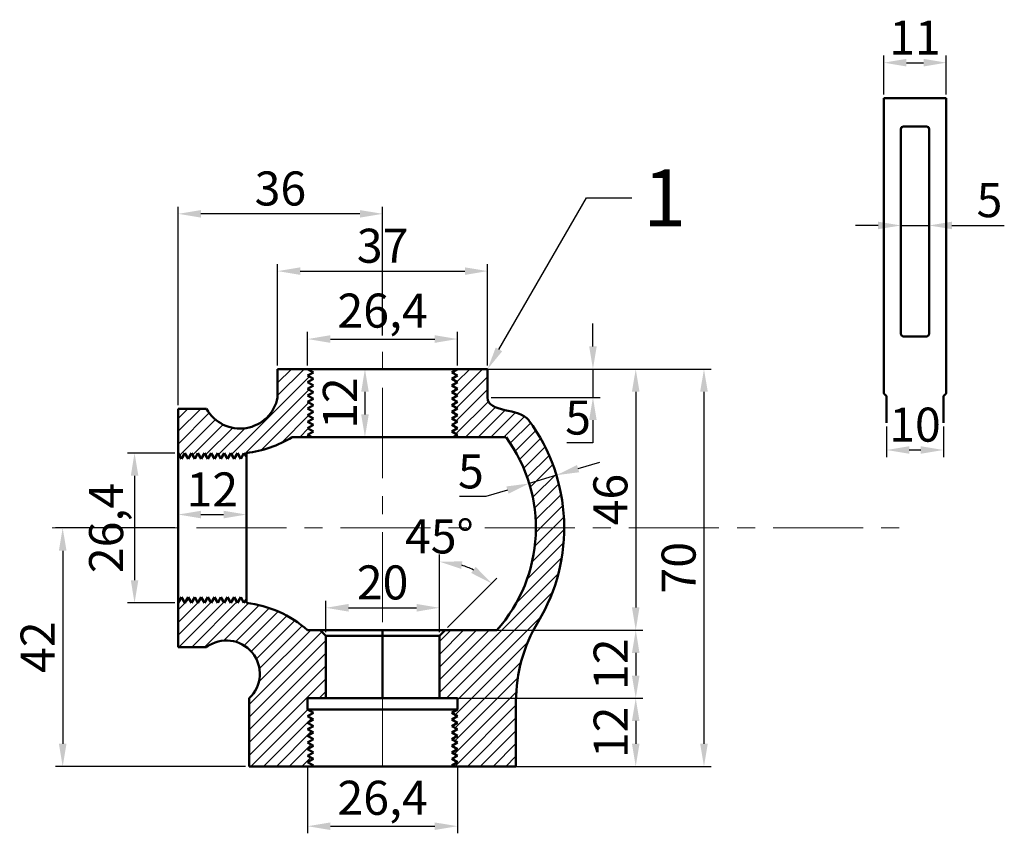
# Model space of a CAD drawing. Units: millimetres. Extents: x -25 to 763, y -62 to 306.
# Tile 3 of 7: x 266 to 439, y 32 to 175. Entities that reach past the tile are written whole.
import ezdxf
from ezdxf import colors
from ezdxf.entities.mleader import LeaderData, LeaderLine
from ezdxf.math import Vec2, Vec3

# ---------------------------------------------------------------- set-up
doc = ezdxf.new("R2010")
doc.units = ezdxf.units.MM
doc.header["$LTSCALE"] = 0.5
doc.linetypes.add('CENTER', pattern=[50.8, 31.75, -6.35, 6.35, -6.35])
for name, color, linetype, lineweight in [('M-CNTR', 1, 'CENTER', 18), ('M-DIMS', 2, 'Continuous', 25), ('M-HATC', 8, 'Continuous', 18), ('M-OUTL', 7, 'Continuous', 50), ('M-TEXT', 3, 'Continuous', 25)]:
    doc.layers.add(name, color=color, linetype=linetype, lineweight=lineweight)
doc.styles.get("Standard").update_dxf_attribs({"font": 'arial.ttf'})
doc.dimstyles.new('ISO-25', dxfattribs={"dimtxt": 6, "dimasz": 4, "dimexe": 1.25, "dimexo": 0.625, "dimtad": 1, "dimtoh": 1, "dimdec": 1, "dimtxsty": 'Standard', "dimcen": 2.5, "dimadec": 0, "dimazin": 0, "dimtfac": 1, "dimtdec": 1, "dimtmove": 0, "dimatfit": 3, "dimfxl": 1, "dimarcsym": 0})

# ---------------------------------------------------------------- blocks, each defined once
blk = doc.blocks.new('*D1')
at = {"layer": 'Defpoints', "color": 0, "ltscale": 0.5, "transparency": 16777216}
for p in [(293.54, 98.87), (285.84, 72.47), (293.54, 72.47)]:
    blk.add_point(p, dxfattribs=at)
at = {"layer": 'M-DIMS', "color": 0, "lineweight": -2, "ltscale": 0.5, "transparency": 16777216}
for p, q in [((292.91, 98.87), (284.59, 98.87)), ((285.84, 94.87), (285.84, 76.47)), ((292.91, 72.47), (284.59, 72.47))]:
    blk.add_line(p, q, dxfattribs=at)
at = {"layer": 'M-DIMS', "color": 0, "ltscale": 0.5, "transparency": 16777216}
for points in [[(285.18, 94.87), (286.51, 94.87), (285.84, 98.87)], [(285.18, 76.47), (286.51, 76.47), (285.84, 72.47)]]:
    blk.add_solid(points, dxfattribs=at)
at = {"layer": 'M-DIMS', "color": 0, "ltscale": 0.5, "transparency": 16777216, "insert": (281.61, 85.67), "char_height": 6, "attachment_point": 5, "rotation": 90}
blk.add_mtext('26,4', dxfattribs=at)
blk = doc.blocks.new('*D2')
at = {"layer": 'Defpoints', "color": 0, "ltscale": 0.5, "transparency": 16777216}
for p in [(293.54, 85.67), (273.18, 43.67), (306.04, 43.67)]:
    blk.add_point(p, dxfattribs=at)
at = {"layer": 'M-DIMS', "color": 0, "lineweight": -2, "ltscale": 0.5, "transparency": 16777216}
for p, q in [((292.91, 85.67), (271.93, 85.67)), ((273.18, 81.67), (273.18, 47.67)), ((305.41, 43.67), (271.93, 43.67))]:
    blk.add_line(p, q, dxfattribs=at)
at = {"layer": 'M-DIMS', "color": 0, "ltscale": 0.5, "transparency": 16777216}
for points in [[(272.51, 81.67), (273.85, 81.67), (273.18, 85.67)], [(272.51, 47.67), (273.85, 47.67), (273.18, 43.67)]]:
    blk.add_solid(points, dxfattribs=at)
at = {"layer": 'M-DIMS', "color": 0, "ltscale": 0.5, "transparency": 16777216, "insert": (269.54, 64.67), "char_height": 6, "attachment_point": 5, "rotation": 90}
blk.add_mtext('42', dxfattribs=at)
blk = doc.blocks.new('*D3')
at = {"layer": 'Defpoints', "color": 0, "ltscale": 0.5, "transparency": 16777216}
for p in [(305.54, 88.04), (293.54, 85.67), (305.54, 85.67)]:
    blk.add_point(p, dxfattribs=at)
at = {"layer": 'M-DIMS', "color": 0, "lineweight": -2, "ltscale": 0.5, "transparency": 16777216}
for p, q in [((293.54, 86.3), (293.54, 89.29)), ((305.54, 86.3), (305.54, 89.29)), ((297.54, 88.04), (301.54, 88.04))]:
    blk.add_line(p, q, dxfattribs=at)
at = {"layer": 'M-DIMS', "color": 0, "ltscale": 0.5, "transparency": 16777216}
for points in [[(297.54, 88.7), (297.54, 87.37), (293.54, 88.04)], [(301.54, 88.7), (301.54, 87.37), (305.54, 88.04)]]:
    blk.add_solid(points, dxfattribs=at)
at = {"layer": 'M-DIMS', "color": 0, "ltscale": 0.5, "transparency": 16777216, "insert": (299.54, 91.68), "char_height": 6, "attachment_point": 5}
blk.add_mtext('12', dxfattribs=at)
blk = doc.blocks.new('*D4')
at = {"layer": 'Defpoints', "color": 0, "ltscale": 0.5, "transparency": 16777216}
for p in [(316.34, 44.4), (342.74, 44.4), (342.74, 33.13)]:
    blk.add_point(p, dxfattribs=at)
at = {"layer": 'M-DIMS', "color": 0, "lineweight": -2, "ltscale": 0.5, "transparency": 16777216}
for p, q in [((316.34, 43.77), (316.34, 31.88)), ((342.74, 43.77), (342.74, 31.88)), ((320.34, 33.13), (338.74, 33.13))]:
    blk.add_line(p, q, dxfattribs=at)
at = {"layer": 'M-DIMS', "color": 0, "ltscale": 0.5, "transparency": 16777216}
for points in [[(320.34, 33.79), (320.34, 32.46), (316.34, 33.13)], [(338.74, 33.79), (338.74, 32.46), (342.74, 33.13)]]:
    blk.add_solid(points, dxfattribs=at)
at = {"layer": 'M-DIMS', "color": 0, "ltscale": 0.5, "transparency": 16777216, "insert": (329.54, 37.36), "char_height": 6, "attachment_point": 5}
blk.add_mtext('26,4', dxfattribs=at)
blk = doc.blocks.new('*D5')
at = {"layer": 'Defpoints', "color": 0, "ltscale": 0.5, "transparency": 16777216}
for p in [(342.74, 55.67), (344.97, 43.67), (374.14, 43.67)]:
    blk.add_point(p, dxfattribs=at)
at = {"layer": 'M-DIMS', "color": 0, "lineweight": -2, "ltscale": 0.5, "transparency": 16777216}
for p, q in [((343.36, 55.67), (375.39, 55.67)), ((374.14, 51.67), (374.14, 47.67)), ((345.6, 43.67), (375.39, 43.67))]:
    blk.add_line(p, q, dxfattribs=at)
at = {"layer": 'M-DIMS', "color": 0, "ltscale": 0.5, "transparency": 16777216}
for points in [[(373.47, 51.67), (374.8, 51.67), (374.14, 55.67)], [(373.47, 47.67), (374.8, 47.67), (374.14, 43.67)]]:
    blk.add_solid(points, dxfattribs=at)
at = {"layer": 'M-DIMS', "color": 0, "ltscale": 0.5, "transparency": 16777216, "insert": (370.5, 49.67), "char_height": 6, "attachment_point": 5, "rotation": 90}
blk.add_mtext('12', dxfattribs=at)
blk = doc.blocks.new('*D6')
at = {"layer": 'Defpoints', "color": 0, "ltscale": 0.5, "transparency": 16777216}
for p in [(339.54, 67.67), (339.54, 55.67), (374.14, 55.67)]:
    blk.add_point(p, dxfattribs=at)
at = {"layer": 'M-DIMS', "color": 0, "lineweight": -2, "ltscale": 0.5, "transparency": 16777216}
for p, q in [((340.16, 67.67), (375.39, 67.67)), ((374.14, 63.67), (374.14, 59.67)), ((340.16, 55.67), (375.39, 55.67))]:
    blk.add_line(p, q, dxfattribs=at)
at = {"layer": 'M-DIMS', "color": 0, "ltscale": 0.5, "transparency": 16777216}
for points in [[(373.47, 63.67), (374.8, 63.67), (374.14, 67.67)], [(373.47, 59.67), (374.8, 59.67), (374.14, 55.67)]]:
    blk.add_solid(points, dxfattribs=at)
at = {"layer": 'M-DIMS', "color": 0, "ltscale": 0.5, "transparency": 16777216, "insert": (370.5, 61.67), "char_height": 6, "attachment_point": 5, "rotation": 90}
blk.add_mtext('12', dxfattribs=at)
blk = doc.blocks.new('*D7')
at = {"layer": 'Defpoints', "color": 0, "ltscale": 0.5, "transparency": 16777216}
for p in [(346.51, 113.67), (346.51, 67.67), (374.14, 67.67)]:
    blk.add_point(p, dxfattribs=at)
at = {"layer": 'M-DIMS', "color": 0, "lineweight": -2, "ltscale": 0.5, "transparency": 16777216}
for p, q in [((347.13, 113.67), (375.39, 113.67)), ((374.14, 109.67), (374.14, 71.67)), ((347.13, 67.67), (375.39, 67.67))]:
    blk.add_line(p, q, dxfattribs=at)
at = {"layer": 'M-DIMS', "color": 0, "ltscale": 0.5, "transparency": 16777216}
for points in [[(373.47, 109.67), (374.8, 109.67), (374.14, 113.67)], [(373.47, 71.67), (374.8, 71.67), (374.14, 67.67)]]:
    blk.add_solid(points, dxfattribs=at)
at = {"layer": 'M-DIMS', "color": 0, "ltscale": 0.5, "transparency": 16777216, "insert": (370.45, 90.67), "char_height": 6, "attachment_point": 5, "rotation": 90}
blk.add_mtext('46', dxfattribs=at)
blk = doc.blocks.new('*D8')
at = {"layer": 'Defpoints', "color": 0, "ltscale": 0.5, "transparency": 16777216}
for p in [(361.26, 113.67), (361.26, 43.67), (386.16, 43.67)]:
    blk.add_point(p, dxfattribs=at)
at = {"layer": 'M-DIMS', "color": 0, "lineweight": -2, "ltscale": 0.5, "transparency": 16777216}
for p, q in [((361.89, 113.67), (387.41, 113.67)), ((386.16, 109.67), (386.16, 47.67)), ((361.89, 43.67), (387.41, 43.67))]:
    blk.add_line(p, q, dxfattribs=at)
at = {"layer": 'M-DIMS', "color": 0, "ltscale": 0.5, "transparency": 16777216}
for points in [[(385.49, 109.67), (386.83, 109.67), (386.16, 113.67)], [(385.49, 47.67), (386.83, 47.67), (386.16, 43.67)]]:
    blk.add_solid(points, dxfattribs=at)
at = {"layer": 'M-DIMS', "color": 0, "ltscale": 0.5, "transparency": 16777216, "insert": (382.47, 78.67), "char_height": 6, "attachment_point": 5, "rotation": 90}
blk.add_mtext('70', dxfattribs=at)
blk = doc.blocks.new('*D9')
at = {"layer": 'Defpoints', "color": 0, "ltscale": 0.5, "transparency": 16777216}
for p in [(360.16, 94.97), (355.37, 93.51), (355.37, 93.51)]:
    blk.add_point(p, dxfattribs=at)
at = {"layer": 'M-DIMS', "color": 0, "lineweight": -2, "ltscale": 0.5, "transparency": 16777216}
for p, q in [((363.98, 96.13), (367.81, 97.29)), ((359.97, 95.57), (359.79, 96.16)), ((355.19, 94.11), (355.01, 94.71)), ((360.16, 94.97), (355.37, 93.51)), ((351.54, 92.35), (347.72, 91.19)), ((347.72, 91.19), (343.11, 91.19))]:
    blk.add_line(p, q, dxfattribs=at)
at = {"layer": 'M-DIMS', "color": 0, "ltscale": 0.5, "transparency": 16777216}
for points in [[(363.79, 96.77), (364.18, 95.49), (360.16, 94.97)], [(351.35, 92.99), (351.74, 91.72), (355.37, 93.51)]]:
    blk.add_solid(points, dxfattribs=at)
at = {"layer": 'M-DIMS', "color": 0, "ltscale": 0.5, "transparency": 16777216, "insert": (345.1, 94.87), "char_height": 6, "attachment_point": 5}
blk.add_mtext('5', dxfattribs=at)
blk = doc.blocks.new('*D10')
at = {"layer": 'Defpoints', "color": 0, "ltscale": 0.5, "transparency": 16777216}
for p in [(339.54, 71.61), (319.54, 66.67), (339.54, 66.67)]:
    blk.add_point(p, dxfattribs=at)
at = {"layer": 'M-DIMS', "color": 0, "lineweight": -2, "ltscale": 0.5, "transparency": 16777216}
for p, q in [((319.54, 67.3), (319.54, 72.86)), ((339.54, 67.3), (339.54, 72.86)), ((323.54, 71.61), (335.54, 71.61))]:
    blk.add_line(p, q, dxfattribs=at)
at = {"layer": 'M-DIMS', "color": 0, "ltscale": 0.5, "transparency": 16777216}
for points in [[(323.54, 72.28), (323.54, 70.94), (319.54, 71.61)], [(335.54, 72.28), (335.54, 70.94), (339.54, 71.61)]]:
    blk.add_solid(points, dxfattribs=at)
at = {"layer": 'M-DIMS', "color": 0, "ltscale": 0.5, "transparency": 16777216, "insert": (329.54, 75.3), "char_height": 6, "attachment_point": 5}
blk.add_mtext('20', dxfattribs=at)
blk = doc.blocks.new('*D11')
at = {"layer": 'Defpoints', "color": 0, "ltscale": 0.5, "transparency": 16777216}
for p in [(346.07, 77.99), (340.54, 67.67), (339.54, 66.67), (339.54, 66.67), (339.54, 55.67)]:
    blk.add_point(p, dxfattribs=at)
at = {"layer": 'M-DIMS', "color": 0, "lineweight": -2, "ltscale": 0.5, "transparency": 16777216}
for p, q in [((339.54, 67.3), (339.54, 80.99)), ((340.98, 68.11), (349.66, 76.8))]:
    blk.add_line(p, q, dxfattribs=at)
blk.add_arc((339.54, 66.67), 13.06, 62.6113, 72.3887, dxfattribs=at)
at = {"layer": 'M-DIMS', "color": 0, "ltscale": 0.5, "transparency": 16777216}
for points in [[(343.39, 78.47), (343.59, 79.78), (339.54, 79.74)], [(345.94, 78.81), (345.15, 77.74), (348.77, 75.91)]]:
    blk.add_solid(points, dxfattribs=at)
at = {"layer": 'M-DIMS', "color": 0, "ltscale": 0.5, "transparency": 16777216, "insert": (339.54, 83.41), "char_height": 6, "attachment_point": 5}
blk.add_mtext('45°', dxfattribs=at)
blk = doc.blocks.new('*D12')
at = {"layer": 'Defpoints', "color": 0, "ltscale": 0.5, "transparency": 16777216}
for p in [(293.54, 141.02), (329.54, 118.96), (293.54, 106.67)]:
    blk.add_point(p, dxfattribs=at)
at = {"layer": 'M-DIMS', "color": 0, "lineweight": -2, "ltscale": 0.5, "transparency": 16777216}
for p, q in [((293.54, 107.3), (293.54, 142.27)), ((329.54, 119.59), (329.54, 142.27)), ((325.54, 141.02), (297.54, 141.02))]:
    blk.add_line(p, q, dxfattribs=at)
at = {"layer": 'M-DIMS', "color": 0, "ltscale": 0.5, "transparency": 16777216}
for points in [[(297.54, 141.68), (297.54, 140.35), (293.54, 141.02)], [(325.54, 141.68), (325.54, 140.35), (329.54, 141.02)]]:
    blk.add_solid(points, dxfattribs=at)
at = {"layer": 'M-DIMS', "color": 0, "ltscale": 0.5, "transparency": 16777216, "insert": (311.54, 144.71), "char_height": 6, "attachment_point": 5}
blk.add_mtext('36', dxfattribs=at)
blk = doc.blocks.new('*D13')
at = {"layer": 'Defpoints', "color": 0, "ltscale": 0.5, "transparency": 16777216}
for p in [(348.04, 130.93), (311.04, 113.67), (348.04, 113.67)]:
    blk.add_point(p, dxfattribs=at)
at = {"layer": 'M-DIMS', "color": 0, "lineweight": -2, "ltscale": 0.5, "transparency": 16777216}
for p, q in [((311.04, 114.3), (311.04, 132.18)), ((348.04, 114.3), (348.04, 132.18)), ((315.04, 130.93), (344.04, 130.93))]:
    blk.add_line(p, q, dxfattribs=at)
at = {"layer": 'M-DIMS', "color": 0, "ltscale": 0.5, "transparency": 16777216}
for points in [[(315.04, 131.59), (315.04, 130.26), (311.04, 130.93)], [(344.04, 131.59), (344.04, 130.26), (348.04, 130.93)]]:
    blk.add_solid(points, dxfattribs=at)
at = {"layer": 'M-DIMS', "color": 0, "ltscale": 0.5, "transparency": 16777216, "insert": (329.54, 134.62), "char_height": 6, "attachment_point": 5}
blk.add_mtext('37', dxfattribs=at)
blk = doc.blocks.new('*D14')
at = {"layer": 'Defpoints', "color": 0, "ltscale": 0.5, "transparency": 16777216}
for p in [(342.74, 118.96), (316.34, 113.67), (342.74, 113.67)]:
    blk.add_point(p, dxfattribs=at)
at = {"layer": 'M-DIMS', "color": 0, "lineweight": -2, "ltscale": 0.5, "transparency": 16777216}
for p, q in [((316.34, 114.3), (316.34, 120.21)), ((342.74, 114.3), (342.74, 120.21)), ((320.34, 118.96), (338.74, 118.96))]:
    blk.add_line(p, q, dxfattribs=at)
at = {"layer": 'M-DIMS', "color": 0, "ltscale": 0.5, "transparency": 16777216}
for points in [[(320.34, 119.63), (320.34, 118.29), (316.34, 118.96)], [(338.74, 119.63), (338.74, 118.29), (342.74, 118.96)]]:
    blk.add_solid(points, dxfattribs=at)
at = {"layer": 'M-DIMS', "color": 0, "ltscale": 0.5, "transparency": 16777216, "insert": (329.54, 123.19), "char_height": 6, "attachment_point": 5}
blk.add_mtext('26,4', dxfattribs=at)
blk = doc.blocks.new('*D15')
at = {"layer": 'Defpoints', "color": 0, "ltscale": 0.5, "transparency": 16777216}
for p in [(329.54, 113.67), (326.43, 101.67), (329.54, 101.67)]:
    blk.add_point(p, dxfattribs=at)
at = {"layer": 'M-DIMS', "color": 0, "lineweight": -2, "ltscale": 0.5, "transparency": 16777216}
for p, q in [((328.91, 113.67), (325.18, 113.67)), ((326.43, 109.67), (326.43, 105.67)), ((328.91, 101.67), (325.18, 101.67))]:
    blk.add_line(p, q, dxfattribs=at)
at = {"layer": 'M-DIMS', "color": 0, "ltscale": 0.5, "transparency": 16777216}
for points in [[(325.77, 109.67), (327.1, 109.67), (326.43, 113.67)], [(325.77, 105.67), (327.1, 105.67), (326.43, 101.67)]]:
    blk.add_solid(points, dxfattribs=at)
at = {"layer": 'M-DIMS', "color": 0, "ltscale": 0.5, "transparency": 16777216, "insert": (322.8, 107.67), "char_height": 6, "attachment_point": 5, "rotation": 90}
blk.add_mtext('12', dxfattribs=at)
blk = doc.blocks.new('*D16')
at = {"layer": 'Defpoints', "color": 0, "ltscale": 0.5, "transparency": 16777216}
for p in [(348.04, 113.67), (348.04, 108.67), (366.6, 108.67)]:
    blk.add_point(p, dxfattribs=at)
at = {"layer": 'M-DIMS', "color": 0, "lineweight": -2, "ltscale": 0.5, "transparency": 16777216}
for p, q in [((366.6, 117.67), (366.6, 121.67)), ((348.66, 113.67), (367.85, 113.67)), ((366.6, 113.67), (366.6, 108.67)), ((348.66, 108.67), (367.85, 108.67)), ((366.6, 104.67), (366.6, 100.67)), ((366.6, 100.67), (361.99, 100.67))]:
    blk.add_line(p, q, dxfattribs=at)
at = {"layer": 'M-DIMS', "color": 0, "ltscale": 0.5, "transparency": 16777216}
for points in [[(365.93, 117.67), (367.26, 117.67), (366.6, 113.67)], [(365.93, 104.67), (367.26, 104.67), (366.6, 108.67)]]:
    blk.add_solid(points, dxfattribs=at)
at = {"layer": 'M-DIMS', "color": 0, "ltscale": 0.5, "transparency": 16777216, "insert": (363.98, 104.35), "char_height": 6, "attachment_point": 5}
blk.add_mtext('5', dxfattribs=at)
blk = doc.blocks.new('*D19')
at = {"layer": 'Defpoints', "color": 0, "ltscale": 0.5, "transparency": 16777216}
for p in [(428.84, 167.65), (417.84, 161.41), (428.84, 161.41)]:
    blk.add_point(p, dxfattribs=at)
at = {"layer": 'M-DIMS', "color": 0, "lineweight": -2, "ltscale": 0.5, "transparency": 16777216}
for p, q in [((417.84, 162.04), (417.84, 168.9)), ((428.84, 162.04), (428.84, 168.9)), ((421.84, 167.65), (424.84, 167.65))]:
    blk.add_line(p, q, dxfattribs=at)
at = {"layer": 'M-DIMS', "color": 0, "ltscale": 0.5, "transparency": 16777216}
for points in [[(421.84, 168.32), (421.84, 166.98), (417.84, 167.65)], [(424.84, 168.32), (424.84, 166.98), (428.84, 167.65)]]:
    blk.add_solid(points, dxfattribs=at)
at = {"layer": 'M-DIMS', "color": 0, "ltscale": 0.5, "transparency": 16777216, "insert": (423.34, 171.29), "char_height": 6, "attachment_point": 5}
blk.add_mtext('11', dxfattribs=at)
blk = doc.blocks.new('*D20')
at = {"layer": 'Defpoints', "color": 0, "ltscale": 0.5, "transparency": 16777216}
for p in [(425.84, 138.97), (420.84, 137.91), (425.84, 137.91)]:
    blk.add_point(p, dxfattribs=at)
at = {"layer": 'M-DIMS', "color": 0, "lineweight": -2, "ltscale": 0.5, "transparency": 16777216}
for p, q in [((416.84, 138.97), (412.84, 138.97)), ((420.84, 138.54), (420.84, 140.22)), ((420.84, 138.97), (425.84, 138.97)), ((425.84, 138.54), (425.84, 140.22)), ((429.84, 138.97), (439.07, 138.97))]:
    blk.add_line(p, q, dxfattribs=at)
at = {"layer": 'M-DIMS', "color": 0, "ltscale": 0.5, "transparency": 16777216}
for points in [[(416.84, 139.64), (416.84, 138.31), (420.84, 138.97)], [(429.84, 139.64), (429.84, 138.31), (425.84, 138.97)]]:
    blk.add_solid(points, dxfattribs=at)
at = {"layer": 'M-DIMS', "color": 0, "ltscale": 0.5, "transparency": 16777216, "insert": (436.46, 142.65), "char_height": 6, "attachment_point": 5}
blk.add_mtext('5', dxfattribs=at)
blk = doc.blocks.new('*D21')
at = {"layer": 'Defpoints', "color": 0, "ltscale": 0.5, "transparency": 16777216}
for p in [(418.34, 104.19), (428.34, 104.19), (428.34, 99.41)]:
    blk.add_point(p, dxfattribs=at)
at = {"layer": 'M-DIMS', "color": 0, "lineweight": -2, "ltscale": 0.5, "transparency": 16777216}
for p, q in [((418.34, 103.57), (418.34, 98.16)), ((428.34, 103.57), (428.34, 98.16)), ((422.34, 99.41), (424.34, 99.41))]:
    blk.add_line(p, q, dxfattribs=at)
at = {"layer": 'M-DIMS', "color": 0, "ltscale": 0.5, "transparency": 16777216}
for points in [[(422.34, 100.08), (422.34, 98.74), (418.34, 99.41)], [(424.34, 100.08), (424.34, 98.74), (428.34, 99.41)]]:
    blk.add_solid(points, dxfattribs=at)
at = {"layer": 'M-DIMS', "color": 0, "ltscale": 0.5, "transparency": 16777216, "insert": (423.34, 103.1), "char_height": 6, "attachment_point": 5}
blk.add_mtext('10', dxfattribs=at)

msp = doc.modelspace()

# ---------------------------------------------------------------- hatches: boundary and pattern name
at = {"layer": 'M-HATC', "ltscale": 0.5}
h = msp.add_hatch(dxfattribs=at)
h.set_pattern_fill('ANSI31', color=256, scale=0.5)
h.paths.add_polyline_path([(305.54, 72.47), (305.54, 73.17), (305.12, 72.47), (304.54, 73.47), (303.97, 72.47), (303.39, 73.47), (302.81, 72.47), (302.24, 73.47), (301.64, 72.47), (301.07, 73.47), (300.49, 72.47), (299.91, 73.47), (299.34, 72.47), (298.76, 73.47), (298.17, 72.47), (297.59, 73.47), (297.01, 72.47), (296.44, 73.47), (295.86, 72.47), (295.28, 73.47), (294.69, 72.47), (294.11, 73.47), (293.54, 72.47), (293.54, 64.67), (298.54, 64.67, -0.948835), (306.04, 55.67), (306.04, 43.67), (317.08, 43.67), (317.34, 43.82), (316.34, 44.4), (317.34, 44.97), (316.34, 45.55), (317.34, 46.13), (316.34, 46.72), (317.34, 47.3), (316.34, 47.87), (317.34, 48.45), (316.34, 49.03), (317.34, 49.61), (316.34, 50.2), (317.34, 50.77), (316.34, 51.35), (317.34, 51.93), (316.34, 52.51), (317.34, 53.08), (316.34, 53.67), (316.34, 55.67), (319.54, 55.67), (319.54, 66.67), (318.54, 67.67), (316.34, 67.67, 0.150651)])
h.paths.add_polyline_path([(302.81, 98.87), (303.39, 97.87), (303.97, 98.87), (304.54, 97.87), (305.12, 98.87), (305.54, 98.17), (305.54, 98.87, 0.107745), (313.61, 101.67), (317.03, 101.67), (316.34, 102.07), (317.34, 102.65), (316.34, 103.24), (317.34, 103.82), (316.34, 104.4), (317.34, 104.97), (316.34, 105.55), (317.34, 106.13), (316.34, 106.72), (317.34, 107.3), (316.34, 107.87), (317.34, 108.45), (316.34, 109.03), (317.34, 109.61), (316.34, 110.2), (317.34, 110.77), (316.34, 111.35), (317.34, 111.93), (316.34, 112.51), (317.34, 113.08), (316.34, 113.67), (311.04, 113.67), (311.04, 108.67, -0.702826), (298.54, 106.67), (293.54, 106.67), (293.54, 98.87), (294.11, 97.87), (294.69, 98.87), (295.28, 97.87), (295.86, 98.87), (296.44, 97.87), (297.01, 98.87), (297.59, 97.87), (298.17, 98.87), (298.76, 97.87), (299.34, 98.87), (299.91, 97.87), (300.49, 98.87), (301.07, 97.87), (301.64, 98.87), (302.24, 97.87)])
edge = h.paths.add_edge_path()
edge.add_arc((329.54, 85.67), 27, 0, 36.3412, ccw=False)
edge.add_line((356.54, 85.67), (361.54, 85.67))
edge.add_arc((329.54, 85.67), 32, 0, 36.3412)
edge.add_spline(control_points=[(355.31, 104.64), (353.67, 106.87), (348.04, 105.9), (348.04, 108.67)], knot_values=[0, 0, 0, 0, 8.320994, 8.320994, 8.320994, 8.320994], degree=3, periodic=0)
edge.add_line((348.04, 108.67), (348.04, 113.67))
edge.add_line((348.04, 113.67), (342.74, 113.67))
edge.add_line((342.74, 113.67), (341.74, 113.08))
edge.add_line((341.74, 113.08), (342.74, 112.51))
edge.add_line((342.74, 112.51), (341.74, 111.93))
edge.add_line((341.74, 111.93), (342.74, 111.35))
edge.add_line((342.74, 111.35), (341.74, 110.77))
edge.add_line((341.74, 110.77), (342.74, 110.2))
edge.add_line((342.74, 110.2), (341.74, 109.61))
edge.add_line((341.74, 109.61), (342.74, 109.03))
edge.add_line((342.74, 109.03), (341.74, 108.45))
edge.add_line((341.74, 108.45), (342.74, 107.87))
edge.add_line((342.74, 107.87), (341.74, 107.3))
edge.add_line((341.74, 107.3), (342.74, 106.72))
edge.add_line((342.74, 106.72), (341.74, 106.13))
edge.add_line((341.74, 106.13), (342.74, 105.55))
edge.add_line((342.74, 105.55), (341.74, 104.97))
edge.add_line((341.74, 104.97), (342.74, 104.4))
edge.add_line((342.74, 104.4), (341.74, 103.82))
edge.add_line((341.74, 103.82), (342.74, 103.24))
edge.add_line((342.74, 103.24), (341.74, 102.65))
edge.add_line((341.74, 102.65), (342.74, 102.07))
edge.add_line((342.74, 102.07), (342.04, 101.67))
edge.add_line((342.04, 101.67), (351.28, 101.67))
h.paths.add_polyline_path([(349.66, 67.67), (340.54, 67.67), (339.54, 66.67), (339.54, 55.67), (342.74, 55.67), (342.74, 53.67), (341.74, 53.08), (342.74, 52.51), (341.74, 51.93), (342.74, 51.35), (341.74, 50.77), (342.74, 50.2), (341.74, 49.61), (342.74, 49.03), (341.74, 48.45), (342.74, 47.87), (341.74, 47.3), (342.74, 46.72), (341.74, 46.13), (342.74, 45.55), (341.74, 44.97), (342.74, 44.4), (341.74, 43.82), (341.99, 43.67), (353.04, 43.67), (353.04, 55.16, -0.136703), (356.93, 69.13, 0.136703), (361.54, 85.67), (356.54, 85.67, -0.184483)])

# ---------------------------------------------------------------- linework, layer by layer
at = {"layer": 'M-CNTR'}
for p, q in [((329.54, 43.67), (329.54, 123.3)), ((271.33, 85.67), (421.69, 85.67))]:
    msp.add_line(p, q, dxfattribs=at)
at = {"layer": 'M-OUTL', "ltscale": 0.5}
for p, q in [((417.84, 161.41), (417.84, 109.58)), ((428.84, 161.41), (417.84, 161.41)), ((428.84, 109.58), (428.84, 161.41)), ((425.34, 156.41), (421.34, 156.41)), ((420.84, 155.91), (420.84, 119.91)), ((425.84, 119.91), (425.84, 155.91)), ((425.34, 119.41), (421.34, 119.41)), ((418.34, 109.08), (418.34, 109.08)), ((418.34, 108.71), (418.34, 104.19)), ((428.34, 109.08), (428.34, 109.08)), ((428.34, 108.71), (428.34, 104.19))]:
    msp.add_line(p, q, dxfattribs=at)
at = {"layer": 'M-OUTL'}
for p, q in [((311.04, 113.67), (348.04, 113.67)), ((311.04, 108.67), (311.04, 113.67)), ((316.34, 113.67), (317.34, 113.08)), ((317.34, 113.08), (316.34, 112.51)), ((342.74, 113.67), (341.74, 113.08)), ((341.74, 113.08), (342.74, 112.51)), ((348.04, 113.67), (348.04, 108.67)), ((316.34, 112.51), (317.34, 111.93)), ((317.34, 111.93), (316.34, 111.35)), ((316.34, 111.35), (317.34, 110.77)), ((342.74, 112.51), (341.74, 111.93)), ((341.74, 111.93), (342.74, 111.35)), ((342.74, 111.35), (341.74, 110.77)), ((317.34, 110.77), (316.34, 110.2)), ((316.34, 110.2), (317.34, 109.61)), ((317.34, 109.61), (316.34, 109.03)), ((341.74, 110.77), (342.74, 110.2)), ((342.74, 110.2), (341.74, 109.61)), ((341.74, 109.61), (342.74, 109.03)), ((316.34, 109.03), (317.34, 108.45)), ((317.34, 108.45), (316.34, 107.87)), ((316.34, 107.87), (317.34, 107.3)), ((342.74, 109.03), (341.74, 108.45)), ((341.74, 108.45), (342.74, 107.87)), ((342.74, 107.87), (341.74, 107.3)), ((293.54, 85.67), (293.54, 106.67)), ((293.54, 106.67), (298.54, 106.67)), ((317.34, 107.3), (316.34, 106.72)), ((316.34, 106.72), (317.34, 106.13)), ((317.34, 106.13), (316.34, 105.55)), ((341.74, 107.3), (342.74, 106.72)), ((342.74, 106.72), (341.74, 106.13)), ((341.74, 106.13), (342.74, 105.55)), ((316.34, 105.55), (317.34, 104.97)), ((317.34, 104.97), (316.34, 104.4)), ((316.34, 104.4), (317.34, 103.82)), ((342.74, 105.55), (341.74, 104.97)), ((341.74, 104.97), (342.74, 104.4)), ((342.74, 104.4), (341.74, 103.82)), ((317.34, 103.82), (316.34, 103.24)), ((316.34, 103.24), (317.34, 102.65)), ((317.34, 102.65), (316.34, 102.07)), ((341.74, 103.82), (342.74, 103.24)), ((342.74, 103.24), (341.74, 102.65)), ((341.74, 102.65), (342.74, 102.07)), ((313.61, 101.67), (351.28, 101.67)), ((316.34, 102.07), (317.03, 101.67)), ((342.74, 102.07), (342.04, 101.67)), ((294.11, 97.87), (293.54, 98.87)), ((294.69, 98.87), (294.11, 97.87)), ((295.28, 97.87), (294.69, 98.87)), ((295.86, 98.87), (295.28, 97.87)), ((296.44, 97.87), (295.86, 98.87)), ((297.01, 98.87), (296.44, 97.87)), ((297.59, 97.87), (297.01, 98.87)), ((298.17, 98.87), (297.59, 97.87)), ((298.76, 97.87), (298.17, 98.87)), ((299.34, 98.87), (298.76, 97.87)), ((299.91, 97.87), (299.34, 98.87)), ((300.49, 98.87), (299.91, 97.87)), ((301.07, 97.87), (300.49, 98.87)), ((301.64, 98.87), (301.07, 97.87)), ((302.24, 97.87), (301.64, 98.87)), ((302.81, 98.87), (302.24, 97.87)), ((303.39, 97.87), (302.81, 98.87)), ((303.97, 98.87), (303.39, 97.87)), ((304.54, 97.87), (303.97, 98.87)), ((305.12, 98.87), (304.54, 97.87)), ((305.54, 98.17), (305.12, 98.87)), ((305.54, 72.47), (305.54, 98.87)), ((293.54, 85.67), (293.54, 64.67)), ((294.11, 73.47), (293.54, 72.47)), ((294.69, 72.47), (294.11, 73.47)), ((295.28, 73.47), (294.69, 72.47)), ((295.86, 72.47), (295.28, 73.47)), ((296.44, 73.47), (295.86, 72.47)), ((297.01, 72.47), (296.44, 73.47)), ((297.59, 73.47), (297.01, 72.47)), ((298.17, 72.47), (297.59, 73.47)), ((298.76, 73.47), (298.17, 72.47)), ((299.34, 72.47), (298.76, 73.47)), ((299.91, 73.47), (299.34, 72.47)), ((300.49, 72.47), (299.91, 73.47)), ((301.07, 73.47), (300.49, 72.47)), ((301.64, 72.47), (301.07, 73.47)), ((302.24, 73.47), (301.64, 72.47)), ((302.81, 72.47), (302.24, 73.47)), ((303.39, 73.47), (302.81, 72.47)), ((303.97, 72.47), (303.39, 73.47)), ((304.54, 73.47), (303.97, 72.47)), ((305.12, 72.47), (304.54, 73.47)), ((305.54, 73.17), (305.12, 72.47)), ((319.54, 67.67), (316.34, 67.67)), ((318.54, 67.67), (339.54, 67.67)), ((319.54, 66.67), (318.54, 67.67)), ((329.54, 67.67), (329.54, 55.67)), ((339.54, 67.67), (349.66, 67.67)), ((339.54, 66.67), (340.54, 67.67)), ((319.54, 66.67), (319.54, 55.67)), ((319.54, 66.67), (339.54, 66.67)), ((339.54, 66.67), (339.54, 55.67)), ((293.54, 64.67), (298.54, 64.67)), ((306.04, 43.67), (306.04, 55.67)), ((316.34, 55.67), (342.74, 55.67)), ((316.34, 55.67), (316.34, 53.67)), ((342.74, 53.67), (342.74, 55.67)), ((353.04, 43.67), (353.04, 55.67)), ((316.34, 53.67), (342.74, 53.67)), ((316.34, 53.67), (317.34, 53.08)), ((317.34, 53.08), (316.34, 52.51)), ((316.34, 52.51), (317.34, 51.93)), ((342.74, 53.67), (341.74, 53.08)), ((341.74, 53.08), (342.74, 52.51)), ((342.74, 52.51), (341.74, 51.93)), ((317.34, 51.93), (316.34, 51.35)), ((316.34, 51.35), (317.34, 50.77)), ((317.34, 50.77), (316.34, 50.2)), ((341.74, 51.93), (342.74, 51.35)), ((342.74, 51.35), (341.74, 50.77)), ((341.74, 50.77), (342.74, 50.2)), ((316.34, 50.2), (317.34, 49.61)), ((317.34, 49.61), (316.34, 49.03)), ((316.34, 49.03), (317.34, 48.45)), ((342.74, 50.2), (341.74, 49.61)), ((341.74, 49.61), (342.74, 49.03)), ((342.74, 49.03), (341.74, 48.45)), ((317.34, 48.45), (316.34, 47.87)), ((316.34, 47.87), (317.34, 47.3)), ((317.34, 47.3), (316.34, 46.72)), ((341.74, 48.45), (342.74, 47.87)), ((342.74, 47.87), (341.74, 47.3)), ((341.74, 47.3), (342.74, 46.72)), ((316.34, 46.72), (317.34, 46.13)), ((317.34, 46.13), (316.34, 45.55)), ((316.34, 45.55), (317.34, 44.97)), ((342.74, 46.72), (341.74, 46.13)), ((341.74, 46.13), (342.74, 45.55)), ((342.74, 45.55), (341.74, 44.97)), ((329.54, 43.67), (306.04, 43.67)), ((317.34, 44.97), (316.34, 44.4)), ((316.34, 44.4), (317.34, 43.82)), ((317.34, 43.82), (317.08, 43.67)), ((329.54, 43.67), (353.04, 43.67)), ((341.74, 44.97), (342.74, 44.4)), ((342.74, 44.4), (341.74, 43.82)), ((341.74, 43.82), (341.99, 43.67))]:
    msp.add_line(p, q, dxfattribs=at)
at = {"layer": 'M-OUTL', "ltscale": 0.5}
for centre, start, end in [((421.34, 155.91), 90, 180), ((425.34, 155.91), 0, 90), ((421.34, 119.91), 180, 270), ((425.34, 119.91), 270, 0), ((418.34, 109.58), 180, 240), ((428.34, 109.58), 300, 0), ((417.84, 108.71), 0, 60), ((428.84, 108.71), 120, 180)]:
    msp.add_arc(centre, 0.5, start, end, dxfattribs=at)
at = {"layer": 'M-OUTL'}
for centre, radius, start, end in [((304.43, 109.92), 6.73, 208.8892, 349.2914), ((329.54, 85.67), 32, 328.8629, 36.3412), ((303.15, 118.79), 20.06, 276.828, 301.4265), ((329.54, 85.67), 27, 318.1897, 36.3412), ((303.15, 52.56), 20.06, 48.903, 83.172), ((380.04, 55.16), 27, 148.8629, 180), ((302.05, 59.98), 5.87, 312.8134, 126.7977)]:
    msp.add_arc(centre, radius, start, end, dxfattribs=at)
msp.add_open_spline([(355.31, 104.64), (353.67, 106.87), (348.04, 105.9), (348.04, 108.67)], degree=3, dxfattribs=at)

# ---------------------------------------------------------------- dimensions: what is measured, and where the dimension line sits
at = {"layer": 'M-DIMS', "ltscale": 0.5}
for base, p1, p2, picture, middle in [((428.84, 167.65), (417.84, 161.41), (428.84, 161.41), '*D19', (423.34, 171.29)), ((425.84, 138.97), (420.84, 137.91), (425.84, 137.91), '*D20', (436.46, 142.65)), ((428.34, 99.41), (418.34, 104.19), (428.34, 104.19), '*D21', (423.34, 103.1)), ((305.54, 88.04), (293.54, 85.67), (305.54, 85.67), '*D3', (299.54, 91.68)), ((339.54, 71.61), (319.54, 66.67), (339.54, 66.67), '*D10', (329.54, 75.3)), ((342.74, 33.13), (316.34, 44.4), (342.74, 44.4), '*D4', (329.54, 37.36))]:
    dim = msp.add_linear_dim(base=base, p1=p1, p2=p2, dimstyle='ISO-25', override={"dimclrd": 0, "dimclre": 0, "dimclrt": 0}, dxfattribs=at)
    dim.commit()
    dim.dimension.update_dxf_attribs({"geometry": picture, "text_midpoint": middle})
for base, p1, p2, picture, middle in [((293.54, 141.02), (329.54, 118.96), (293.54, 106.67), '*D12', (311.54, 141.02)), ((348.04, 130.93), (311.04, 113.67), (348.04, 113.67), '*D13', (329.54, 130.93)), ((342.74, 118.96), (316.34, 113.67), (342.74, 113.67), '*D14', (329.54, 118.96))]:
    dim = msp.add_linear_dim(base=base, p1=p1, p2=p2, dimstyle='ISO-25', override={"dimclrd": 0, "dimclre": 0, "dimclrt": 0}, dxfattribs=at)
    dim.commit()
    dim.dimension.update_dxf_attribs({"geometry": picture, "text_midpoint": middle, "dimtype": 160})
for base, p1, p2, override, picture, middle in [((366.6, 108.67), (348.04, 113.67), (348.04, 108.67), {"dimclrd": 0, "dimclre": 0, "dimclrt": 0}, '*D16', (363.98, 104.35)), ((326.43, 101.67), (329.54, 113.67), (329.54, 101.67), {"dimclrd": 0, "dimclre": 0, "dimclrt": 0}, '*D15', (322.8, 107.67)), ((374.14, 67.67), (346.51, 113.67), (346.51, 67.67), {"dimclrd": 0, "dimclre": 0, "dimclrt": 0, "dimtmove": 0}, '*D7', (370.45, 90.67)), ((386.16, 43.67), (361.26, 113.67), (361.26, 43.67), {"dimclrd": 0, "dimclre": 0, "dimclrt": 0}, '*D8', (382.47, 78.67)), ((285.84, 72.47), (293.54, 98.87), (293.54, 72.47), {"dimclrd": 0, "dimclre": 0, "dimclrt": 0}, '*D1', (281.61, 85.67))]:
    dim = msp.add_linear_dim(base=base, p1=p1, p2=p2, angle=90, dimstyle='ISO-25', override=override, dxfattribs=at)
    dim.commit()
    dim.dimension.update_dxf_attribs({"geometry": picture, "text_midpoint": middle})
dim = msp.add_aligned_dim(p1=(360.16, 94.97), p2=(355.37, 93.51), distance=0, dimstyle='ISO-25', override={"dimclrd": 0, "dimclre": 0, "dimclrt": 0}, dxfattribs=at)
dim.commit()
dim.dimension.update_dxf_attribs({"geometry": '*D9', "text_midpoint": (345.1, 94.87)})
dim = msp.add_angular_dim_2l(base=(346.07, 77.99), line1=((339.54, 66.67), (339.54, 55.67)), line2=((339.54, 66.67), (340.54, 67.67)), dimstyle='ISO-25', override={"dimclrd": 0, "dimclre": 0, "dimclrt": 0}, dxfattribs=at)
dim.commit()
dim.dimension.update_dxf_attribs({"geometry": '*D11', "text_midpoint": (339.54, 79.74), "dimtype": 162})
for base, p1, p2, override, picture, middle in [((273.18, 43.67), (293.54, 85.67), (306.04, 43.67), {"dimclrd": 0, "dimclre": 0, "dimclrt": 0}, '*D2', (273.18, 64.67)), ((374.14, 55.67), (339.54, 67.67), (339.54, 55.67), {"dimclrd": 0, "dimclre": 0, "dimclrt": 0, "dimtmove": 0}, '*D6', (374.14, 61.67)), ((374.14, 43.67), (342.74, 55.67), (344.97, 43.67), {"dimclrd": 0, "dimclre": 0, "dimclrt": 0, "dimtmove": 0}, '*D5', (374.14, 49.67))]:
    dim = msp.add_linear_dim(base=base, p1=p1, p2=p2, angle=90, dimstyle='ISO-25', override=override, dxfattribs=at)
    dim.commit()
    dim.dimension.update_dxf_attribs({"geometry": picture, "text_midpoint": middle, "dimtype": 160})

# ---------------------------------------------------------------- leaders
at = {"layer": 'M-TEXT', "ltscale": 0.5}
ml = msp.add_multileader_mtext('Standard', dxfattribs=at)
ml.set_content('1', color=256)
ml.set_leader_properties()
ml.build(insert=Vec2(0, 0))
ctx = ml.context
ctx.base_point, ctx.char_height, ctx.plane_origin = Vec3(373.45, 143.83), 10, Vec3(348.04, 113.67)
notes = []
notes.append((ctx, [(0, (1, 1, 0), (365.45, 143.83), (1, 0), 8, [(0, [(348.04, 113.67)], 0, [])])]))
ctx.mtext.insert, ctx.mtext.flow_direction = Vec3(375.45, 148.83), 5
for ctx, leaders in notes:
    for number, flags, end, landing, length, lines in leaders:
        leader = LeaderData()
        leader.index, (leader.has_last_leader_line, leader.has_dogleg_vector, leader.attachment_direction) = number, flags
        leader.last_leader_point, leader.dogleg_vector, leader.dogleg_length = Vec3(end), Vec3(landing), length
        for number, points, colour, breaks in lines:
            line = LeaderLine()
            line.index, line.vertices, line.color, line.breaks = number, Vec3.list(points), colors.encode_raw_color(colour), breaks
            leader.lines.append(line)
        ctx.leaders.append(leader)

doc.saveas('drawing.dxf')
